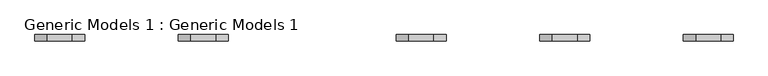
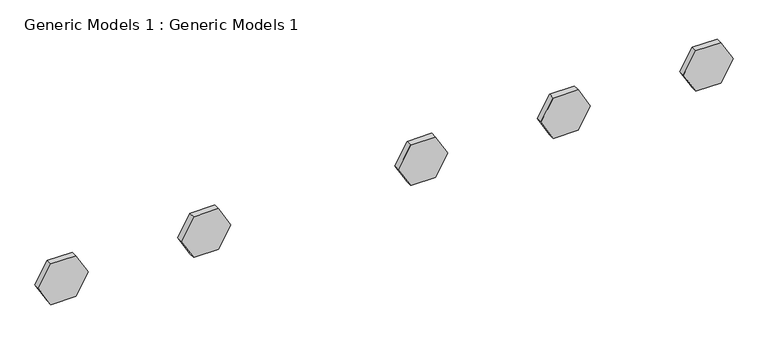
"""IFC4 building model written with IfcOpenShell, lengths in millimetres: proxy geometry, Generic Models 1 : Generic Models 1."""

from ifc_helpers import new_model, si_unit, frame, origin, place, context, project, spatial, polyline, outline, extrude, source, transform, mapped, element, save


def generic_models_1_generic_models_1_ff25953a(model_context):
    return source(origin(), model_context, "Body", "SweptSolid", [
        extrude(outline(polyline([(1292.9011215, -8285.8180218), (1292.9011215, -8895.4180218), (764.9720354, -9200.2180218), (237.0429492, -8895.4180218), (237.0429492, -8285.8180218), (764.9720354, -7981.0180218), (1292.9011215, -8285.8180218)])), frame((0.0, -14006.2284905, 0.0), z_axis=(0.0, 1.0, 0.0), x_axis=(0.0, 0.0, 1.0)), (0.0, 0.0, 1.0), 152.4),
        extrude(outline(polyline([(1292.9011215, -4780.6180218), (1292.9011215, -5390.2180218), (764.9720354, -5695.0180218), (237.0429492, -5390.2180218), (237.0429492, -4780.6180218), (764.9720354, -4475.8180218), (1292.9011215, -4780.6180218)])), frame((0.0, -14006.2284905, 0.0), z_axis=(0.0, 1.0, 0.0), x_axis=(0.0, 0.0, 1.0)), (0.0, 0.0, 1.0), 152.4),
        extrude(outline(polyline([(1292.9011215, 553.3819782), (1292.9011215, -56.2180218), (764.9720354, -361.0180218), (237.0429492, -56.2180218), (237.0429492, 553.3819782), (764.9720354, 858.1819782), (1292.9011215, 553.3819782)])), frame((0.0, -14006.2284905, 0.0), z_axis=(0.0, 1.0, 0.0), x_axis=(0.0, 0.0, 1.0)), (0.0, 0.0, 1.0), 152.4),
        extrude(outline(polyline([(1292.9011215, 4058.5819782), (1292.9011215, 3448.9819782), (764.9720354, 3144.1819782), (237.0429492, 3448.9819782), (237.0429492, 4058.5819782), (764.9720354, 4363.3819782), (1292.9011215, 4058.5819782)])), frame((0.0, -14006.2284905, 0.0), z_axis=(0.0, 1.0, 0.0), x_axis=(0.0, 0.0, 1.0)), (0.0, 0.0, 1.0), 152.4),
        extrude(outline(polyline([(1292.9011215, 7563.7819782), (1292.9011215, 6954.1819782), (764.9720354, 6649.3819782), (237.0429492, 6954.1819782), (237.0429492, 7563.7819782), (764.9720354, 7868.5819782), (1292.9011215, 7563.7819782)])), frame((0.0, -14006.2284905, 0.0), z_axis=(0.0, 1.0, 0.0), x_axis=(0.0, 0.0, 1.0)), (0.0, 0.0, 1.0), 152.4),
    ])


if __name__ == "__main__":
    model = new_model("IFC4")
    model_context = context("Model", 3, world=origin())
    ifc_project = project(units=[si_unit("LENGTHUNIT", "METRE", prefix="MILLI")], contexts=[model_context])
    site = spatial("IfcSite", under=ifc_project)
    building = spatial("IfcBuilding", under=site)
    placement = place(None, origin())
    generic_models_1_generic_models_1_shape = generic_models_1_generic_models_1_ff25953a(model_context)
    element("IfcBuildingElementProxy", 1, Name="Generic Models 1 : Generic Models 1", ObjectType="Generic Models 1 : Generic Models 1", at=placement, inside=building, context=model_context, shape_type="MappedRepresentation", body=[
        mapped(generic_models_1_generic_models_1_shape, transform((0.0, 0.0, 0.0), x_axis=(1.0, 0.0, 0.0), y_axis=(0.0, 1.0, 0.0), z_axis=(0.0, 0.0, 1.0))),
    ])
    save(model, "model.ifc")

# Revit data of these elements
# Element 1 (IfcBuildingElementProxy, "Generic Models 1 : Generic Models 1")
#   Materials on its faces: "Brick, Common"
# Materials
#   "Brick, Common": class "Masonry", colour RGB 170 98 104, transparency 0, Description = "Common brick", Cost = 0
